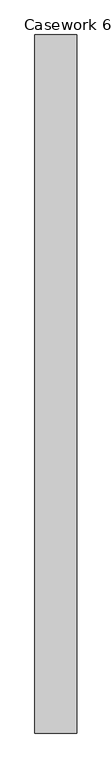
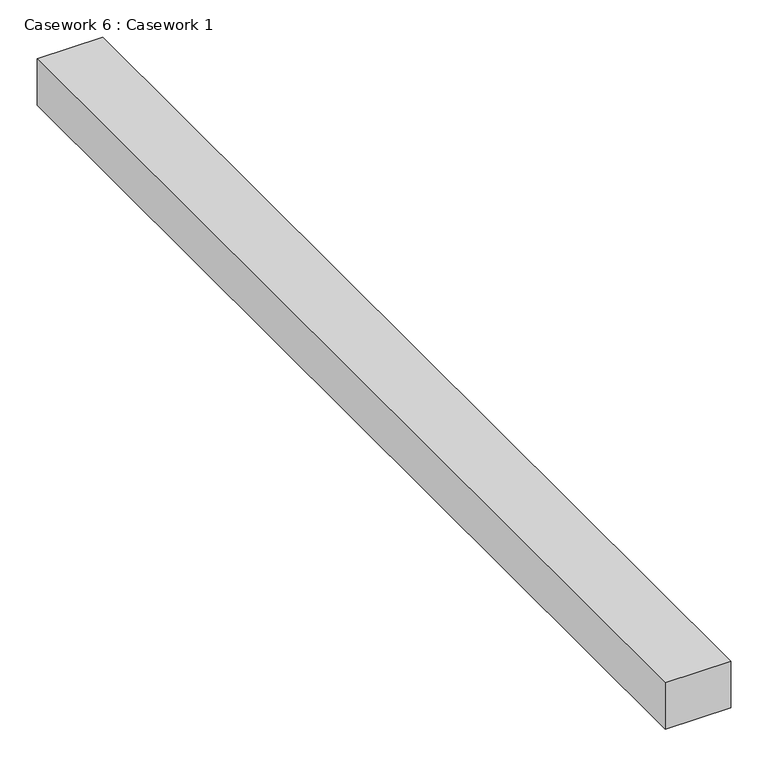
"""IFC4 building model written with IfcOpenShell, lengths in millimetres: furniture geometry, Casework 6 : Casework 1."""

from ifc_helpers import new_model, si_unit, frame, origin, place, context, project, spatial, polyline, outline, extrude, source, transform, mapped, element, save


def casework_6_casework_1_aba422e7(model_context):
    return source(origin(), model_context, "Body", "SweptSolid", [
        extrude(outline(polyline([(8138.5559589, 14787.9496924), (8138.5559589, 13098.8496924), (8036.9559589, 13098.8496924), (8036.9559589, 14787.9496924), (8138.5559589, 14787.9496924)])), frame((0.0, 0.0, 3581.4), z_axis=(0.0, 0.0, 1.0), x_axis=(1.0, 0.0, 0.0)), (0.0, 0.0, 1.0), 76.2),
    ])


if __name__ == "__main__":
    model = new_model("IFC4")
    model_context = context("Model", 3, world=origin())
    ifc_project = project(units=[si_unit("LENGTHUNIT", "METRE", prefix="MILLI")], contexts=[model_context])
    site = spatial("IfcSite", under=ifc_project)
    building = spatial("IfcBuilding", under=site)
    placement = place(None, origin())
    casework_6_casework_1_shape = casework_6_casework_1_aba422e7(model_context)
    element("IfcFurniture", 1, ObjectType="Casework 6 : Casework 1", at=placement, inside=building, context=model_context, shape_type="MappedRepresentation", body=[
        mapped(casework_6_casework_1_shape, transform((0.0, 0.0, 0.0), x_axis=(1.0, 0.0, 0.0), y_axis=(0.0, 1.0, 0.0), z_axis=(0.0, 0.0, 1.0))),
    ])
    save(model, "model.ifc")

# Revit data of these elements
# Element 1 (IfcFurniture, "Casework 6 : Casework 1")
#   Materials on its faces: "Clad - White"
# Materials
#   "Clad - White": class "Wood", colour RGB 242 242 238, transparency 0, Cost = 0
